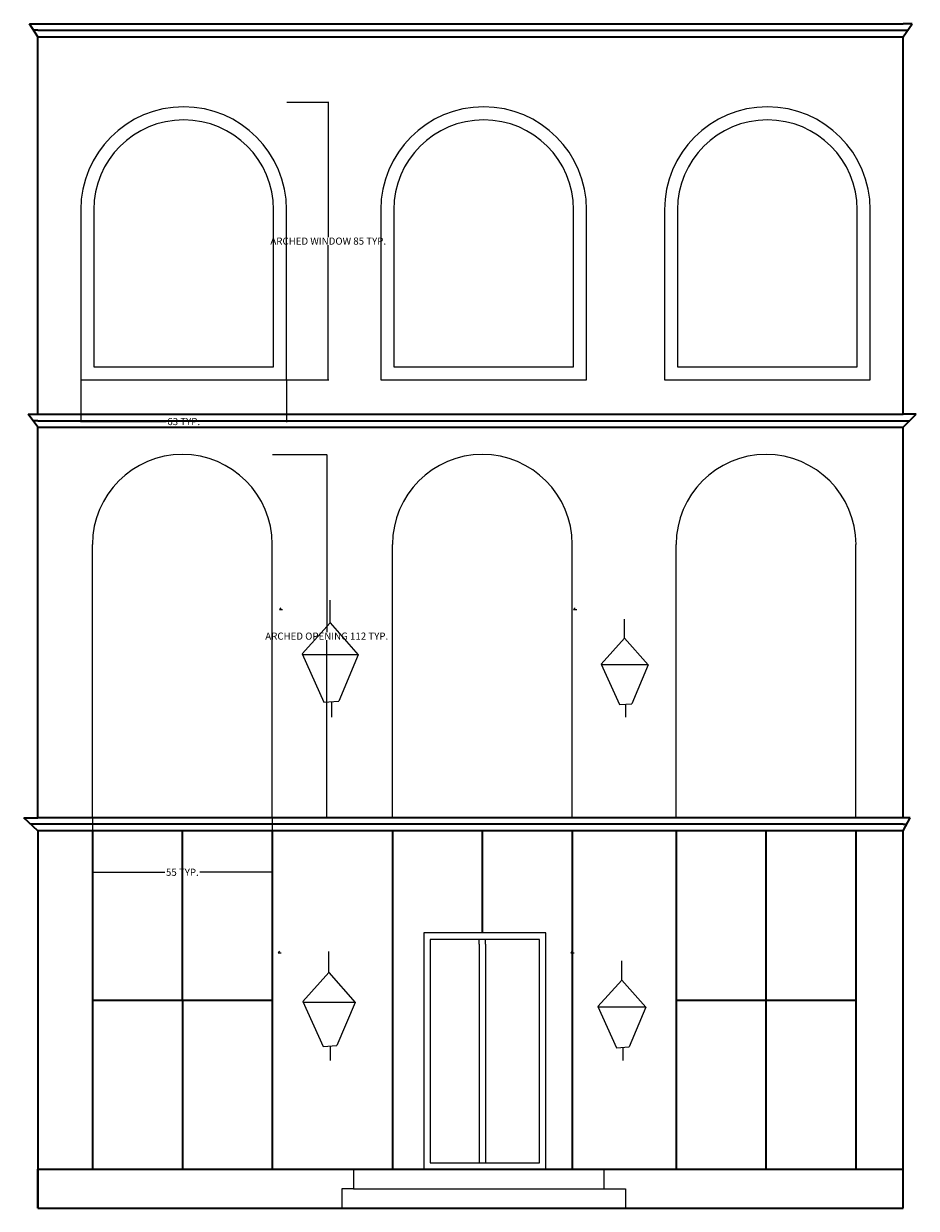
# Model space of a CAD drawing. Units: inches. Extents: x 8 to 283, y 106 to 470.
import ezdxf

# ---------------------------------------------------------------- set-up
doc = ezdxf.new("R2010")
doc.units = ezdxf.units.IN
doc.header["$MEASUREMENT"] = 0
for name, color, linetype, lineweight in [('A-ANNO-DIMS', 2, 'Continuous', 18), ('A-DOOR', 3, 'Continuous', 25), ('A-ELEV', 7, 'Continuous', 35), ('A-FLOR-STRS', 2, 'Continuous', 25), ('A-GLAZ', 4, 'Continuous', 25), ('E-LITE', 6, 'Continuous', 18)]:
    doc.layers.add(name, color=color, linetype=linetype, lineweight=lineweight)
doc.styles.get("Standard").update_dxf_attribs({"font": 'arial.ttf'})
doc.dimstyles.get("Standard").update_dxf_attribs({"dimtxt": 2.1875, "dimasz": 0.18, "dimexe": 0.18, "dimexo": 0.0625, "dimgap": 0.09, "dimtad": 0, "dimtih": 1, "dimtoh": 1, "dimdec": 4, "dimzin": 0, "dimdsep": 46, "dimlunit": 4, "dimtxsty": 'Standard', "dimcen": 0.09, "dimadec": 0, "dimazin": 0, "dimtfac": 1, "dimtdec": 4, "dimtofl": 0, "dimtmove": 0, "dimatfit": 3, "dimfxl": 1, "dimtolj": 1, "dimtzin": 0, "dimarcsym": 0})

# ---------------------------------------------------------------- blocks, each defined once
blk = doc.blocks.new('WIN-ARCHED')
for points in [[(63.27, 52.16, 1), (0.02, 52.16), (0.02, -0.11), (63.27, -0.11)], [(59.27, 52.16, 1), (4.02, 52.16), (4.02, 3.89), (59.27, 3.89)]]:
    blk.add_lwpolyline(points, format="xyb", close=True)
blk = doc.blocks.new('ARCH-OPENING')
for p, q in [((0, 0), (0, 84)), ((55.25, 0), (55.25, 84))]:
    blk.add_line(p, q)
blk.add_arc((27.63, 84), 27.63, 0, 180)
blk = doc.blocks.new('*D3')
at = {"layer": 'A-ANNO-DIMS', "color": 0, "lineweight": -2, "transparency": 16777216}
for p, q in [((89.34, 446.2), (102.25, 446.2)), ((102.07, 446.02), (102.07, 404.77)), ((102.07, 361.07), (102.07, 402.32)), ((89.34, 360.89), (102.25, 360.89))]:
    blk.add_line(p, q, dxfattribs=at)
at = {"layer": 'A-ANNO-DIMS', "color": 0, "transparency": 16777216}
for points in [[(102.04, 446.02), (102.1, 446.02), (102.07, 446.2)], [(102.04, 361.07), (102.1, 361.07), (102.07, 360.89)]]:
    blk.add_solid(points, dxfattribs=at)
at = {"layer": 'Defpoints', "color": 0, "transparency": 16777216}
for p in [(89.27, 446.2), (102.07, 446.2), (89.27, 360.89)]:
    blk.add_point(p, dxfattribs=at)
at = {"layer": 'A-ANNO-DIMS', "color": 0, "transparency": 16777216, "insert": (102.07, 403.55), "char_height": 2.1875, "attachment_point": 5}
blk.add_mtext('\\A1;ARCHED WINDOW 85 TYP.', dxfattribs=at)
blk = doc.blocks.new('*D4')
at = {"layer": 'A-ANNO-DIMS', "color": 0, "lineweight": -2, "transparency": 16777216}
for p, q in [((26.02, 360.83), (26.02, 347.92)), ((89.27, 360.83), (89.27, 347.92)), ((26.2, 348.1), (52.23, 348.1)), ((89.09, 348.1), (63.07, 348.1))]:
    blk.add_line(p, q, dxfattribs=at)
at = {"layer": 'A-ANNO-DIMS', "color": 0, "transparency": 16777216}
for points in [[(26.2, 348.13), (26.2, 348.07), (26.02, 348.1)], [(89.09, 348.13), (89.09, 348.07), (89.27, 348.1)]]:
    blk.add_solid(points, dxfattribs=at)
at = {"layer": 'Defpoints', "color": 0, "transparency": 16777216}
for p in [(26.02, 360.89), (89.27, 360.89), (89.27, 348.1)]:
    blk.add_point(p, dxfattribs=at)
at = {"layer": 'A-ANNO-DIMS', "color": 0, "transparency": 16777216, "insert": (57.65, 348.1), "char_height": 2.1875, "attachment_point": 5}
blk.add_mtext('\\A1;63 TYP.', dxfattribs=at)
blk = doc.blocks.new('*D5')
at = {"layer": 'A-ANNO-DIMS', "color": 0, "lineweight": -2, "transparency": 16777216}
for p, q in [((84.93, 337.98), (101.79, 337.98)), ((101.61, 337.8), (101.61, 283.39)), ((101.61, 226.53), (101.61, 280.95)), ((84.93, 226.35), (101.79, 226.35))]:
    blk.add_line(p, q, dxfattribs=at)
at = {"layer": 'A-ANNO-DIMS', "color": 0, "transparency": 16777216}
for points in [[(101.58, 337.8), (101.64, 337.8), (101.61, 337.98)], [(101.58, 226.53), (101.64, 226.53), (101.61, 226.35)]]:
    blk.add_solid(points, dxfattribs=at)
at = {"layer": 'Defpoints', "color": 0, "transparency": 16777216}
for p in [(84.87, 337.98), (101.61, 337.98), (84.87, 226.35)]:
    blk.add_point(p, dxfattribs=at)
at = {"layer": 'A-ANNO-DIMS', "color": 0, "transparency": 16777216, "insert": (101.61, 282.17), "char_height": 2.1875, "attachment_point": 5}
blk.add_mtext('\\A1;ARCHED OPENING 112 TYP.', dxfattribs=at)
blk = doc.blocks.new('*D6')
at = {"layer": 'A-ANNO-DIMS', "color": 0, "lineweight": -2, "transparency": 16777216}
for p, q in [((29.62, 226.29), (29.62, 209.43)), ((84.87, 226.29), (84.87, 209.43)), ((29.8, 209.61), (51.83, 209.61)), ((84.69, 209.61), (62.66, 209.61))]:
    blk.add_line(p, q, dxfattribs=at)
at = {"layer": 'A-ANNO-DIMS', "color": 0, "transparency": 16777216}
for points in [[(29.8, 209.64), (29.8, 209.58), (29.62, 209.61)], [(84.69, 209.64), (84.69, 209.58), (84.87, 209.61)]]:
    blk.add_solid(points, dxfattribs=at)
at = {"layer": 'Defpoints', "color": 0, "transparency": 16777216}
for p in [(29.62, 226.35), (84.87, 226.35), (84.87, 209.61)]:
    blk.add_point(p, dxfattribs=at)
at = {"layer": 'A-ANNO-DIMS', "color": 0, "transparency": 16777216, "insert": (57.24, 209.61), "char_height": 2.1875, "attachment_point": 5}
blk.add_mtext('\\A1;55 TYP.', dxfattribs=at)

msp = doc.modelspace()

# ---------------------------------------------------------------- linework, layer by layer
at = {"layer": 'A-DOOR'}
for p, q in [((148.45, 187.56), (148.45, 188.99)), ((148.45, 187.56), (148.45, 120.35)), ((150.45, 187.56), (150.45, 188.99)), ((150.45, 187.56), (150.45, 120.35))]:
    msp.add_line(p, q, dxfattribs=at)
for points in [[(131.42, 118.35), (168.98, 118.35), (168.98, 190.99), (131.42, 190.99)], [(133.42, 120.35), (166.98, 120.35), (166.98, 188.99), (133.42, 188.99)]]:
    msp.add_lwpolyline(points, close=True, dxfattribs=at)
at = {"layer": 'A-ELEV'}
for p, q in [((12.83, 466.35), (10.26, 470.35)), ((10.26, 470.35), (12.83, 470.35)), ((12.83, 470.35), (278.79, 470.35)), ((278.79, 466.35), (281.53, 470.35)), ((281.53, 470.35), (278.79, 470.35)), ((12.83, 468.35), (11.54, 468.35)), ((12.83, 468.35), (278.79, 468.35)), ((12.83, 350.35), (12.83, 466.35)), ((12.83, 466.35), (278.79, 466.35)), ((278.79, 468.35), (280.16, 468.35)), ((278.79, 350.35), (278.79, 466.35)), ((12.83, 346.35), (9.82, 350.35)), ((9.82, 350.35), (12.83, 350.35)), ((12.83, 350.35), (278.79, 350.35)), ((278.79, 346.35), (282.82, 350.35)), ((282.82, 350.35), (278.79, 350.35)), ((12.83, 348.35), (11.32, 348.35)), ((12.83, 348.35), (278.79, 348.35)), ((12.83, 226.35), (12.83, 346.35)), ((12.83, 346.35), (278.79, 346.35)), ((278.79, 348.35), (280.8, 348.35)), ((278.79, 226.35), (278.79, 346.35)), ((12.83, 222.35), (8.48, 226.35)), ((8.48, 226.35), (12.83, 226.35)), ((278.79, 226.35), (12.83, 226.35)), ((278.79, 222.35), (280.95, 226.35)), ((280.95, 226.35), (278.79, 226.35)), ((12.83, 224.35), (10.65, 224.35)), ((278.79, 224.35), (12.83, 224.35)), ((12.83, 222.35), (12.83, 106.35)), ((278.79, 222.35), (12.83, 222.35)), ((29.62, 222.35), (29.62, 118.35)), ((57.24, 170.35), (57.24, 222.35)), ((84.87, 222.35), (84.87, 118.35)), ((121.83, 222.35), (121.83, 118.35)), ((149.45, 190.99), (149.45, 222.35)), ((149.45, 190.99), (149.45, 222.35)), ((177.08, 222.35), (177.08, 118.35)), ((209.02, 222.35), (209.02, 118.35)), ((236.65, 118.35), (236.65, 222.35)), ((236.65, 170.35), (236.65, 222.35)), ((264.27, 222.35), (264.27, 118.35)), ((278.79, 224.35), (279.87, 224.35)), ((278.79, 106.35), (278.79, 222.35)), ((29.62, 170.35), (84.87, 170.35)), ((57.24, 170.35), (57.24, 118.35)), ((209.02, 170.35), (264.27, 170.35)), ((12.83, 106.35), (12.83, 118.35)), ((12.83, 118.35), (278.79, 118.35)), ((12.83, 106.35), (64.31, 106.35)), ((64.31, 106.35), (278.79, 106.35))]:
    msp.add_line(p, q, dxfattribs=at)
at = {"layer": 'A-FLOR-STRS'}
for p, q in [((121.83, 118.35), (109.83, 118.35)), ((109.83, 118.35), (109.83, 112.35)), ((186.9, 112.35), (186.9, 118.35)), ((109.83, 112.35), (106.25, 112.35)), ((106.25, 112.35), (106.25, 106.35)), ((109.83, 112.35), (186.9, 112.35)), ((186.9, 112.35), (193.42, 112.35)), ((193.42, 112.35), (193.42, 106.35))]:
    msp.add_line(p, q, dxfattribs=at)
at = {"layer": 'A-GLAZ'}
for points in [[(118.23, 360.89), (181.48, 360.89), (181.48, 413.16, 1), (118.23, 413.16)], [(122.23, 364.89), (177.48, 364.89), (177.48, 413.16, 1), (122.23, 413.16)]]:
    msp.add_lwpolyline(points, format="xyb", close=True, dxfattribs=at)
at = {"layer": 'E-LITE'}
for p, q in [((102.68, 286.27), (102.68, 293.25)), ((87.5, 290.84), (87.05, 290.32)), ((87.05, 290.32), (88.06, 290.32)), ((177.92, 290.84), (177.47, 290.32)), ((177.47, 290.32), (178.49, 290.32)), ((102.68, 286.27), (94.03, 276.73)), ((102.68, 286.27), (111.32, 276.43)), ((193.16, 281.54), (193.16, 287.39)), ((193.16, 281.54), (185.92, 273.56)), ((193.16, 281.54), (200.4, 273.31)), ((94.03, 276.73), (100.77, 261.87)), ((102.68, 276.43), (94.36, 276.43)), ((111.32, 276.43), (102.68, 276.43)), ((111.32, 276.43), (105.33, 262.15)), ((185.92, 273.56), (191.57, 261.12)), ((193.16, 273.31), (186.2, 273.31)), ((200.4, 273.31), (193.16, 273.31)), ((200.4, 273.31), (195.38, 261.35)), ((100.77, 261.87), (105.33, 262.15)), ((103.05, 262.01), (103.05, 257.25)), ((191.57, 261.12), (195.38, 261.35)), ((193.48, 261.24), (193.48, 257.25)), ((87.08, 185.36), (86.64, 184.84)), ((86.64, 184.84), (87.65, 184.84)), ((102.29, 178.8), (102.29, 185.31)), ((177.09, 185.36), (176.64, 184.84)), ((176.64, 184.84), (177.66, 184.84)), ((192.33, 176.48), (192.33, 182.43)), ((102.29, 178.8), (94.24, 169.92)), ((102.29, 178.8), (110.35, 169.64)), ((192.33, 176.48), (184.96, 168.36)), ((192.33, 176.48), (199.69, 168.11)), ((94.24, 169.92), (100.52, 156.07)), ((102.29, 169.64), (94.54, 169.64)), ((110.35, 169.64), (102.29, 169.64)), ((110.35, 169.64), (104.76, 156.34)), ((184.96, 168.36), (190.71, 155.7)), ((192.33, 168.11), (185.24, 168.11)), ((199.69, 168.11), (192.33, 168.11)), ((199.69, 168.11), (194.59, 155.95)), ((100.52, 156.07), (104.76, 156.34)), ((102.64, 156.21), (102.64, 151.77)), ((190.71, 155.7), (194.59, 155.95)), ((192.65, 155.82), (192.65, 151.77))]:
    msp.add_line(p, q, dxfattribs=at)

# ---------------------------------------------------------------- block references
at = {"layer": 'A-GLAZ'}
for name, p in [('WIN-ARCHED', (26, 361)), ('WIN-ARCHED', (205.4, 361)), ('ARCH-OPENING', (29.62, 226.35)), ('ARCH-OPENING', (121.83, 226.35)), ('ARCH-OPENING', (209.02, 226.35))]:
    msp.add_blockref(name, p, dxfattribs=at)

# ---------------------------------------------------------------- dimensions: what is measured, and where the dimension line sits
at = {"layer": 'A-ANNO-DIMS'}
for base, p1, p2, text, picture, middle in [((102.07, 446.2), (89.27, 360.89), (89.27, 446.2), 'ARCHED WINDOW <> TYP.', '*D3', (102.07, 403.55)), ((101.61, 337.98), (84.87, 226.35), (84.87, 337.98), 'ARCHED OPENING <> TYP.', '*D5', (101.61, 282.17))]:
    dim = msp.add_linear_dim(base=base, p1=p1, p2=p2, angle=90, text=text, dimstyle='Standard', override={"dimdec": 0, "dimlfac": 1, "dimrnd": 0, "dimzin": 0, "dimdsep": 46, "dimlunit": 2}, dxfattribs=at)
    dim.commit()
    dim.dimension.update_dxf_attribs({"geometry": picture, "text_midpoint": middle})
for base, p1, p2, picture, middle in [((89.27, 348.1), (26.02, 360.89), (89.27, 360.89), '*D4', (57.65, 348.1)), ((84.87, 209.61), (29.62, 226.35), (84.87, 226.35), '*D6', (57.24, 209.61))]:
    dim = msp.add_linear_dim(base=base, p1=p1, p2=p2, text='<> TYP.', dimstyle='Standard', override={"dimdec": 0, "dimlfac": 1, "dimrnd": 0, "dimzin": 0, "dimdsep": 46, "dimlunit": 2}, dxfattribs=at)
    dim.commit()
    dim.dimension.update_dxf_attribs({"geometry": picture, "text_midpoint": middle})

doc.saveas('drawing.dxf')
